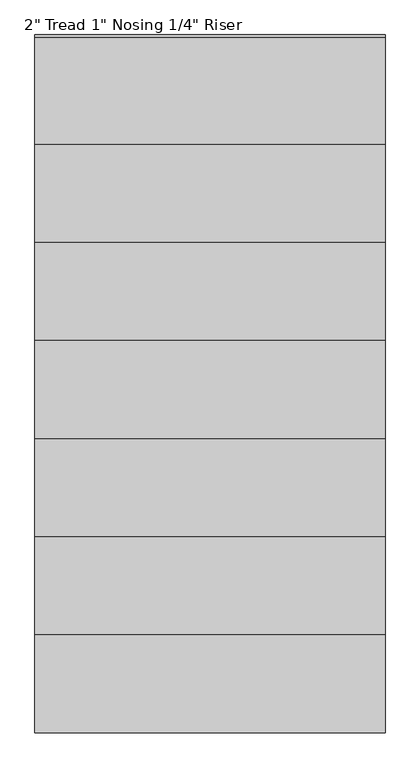
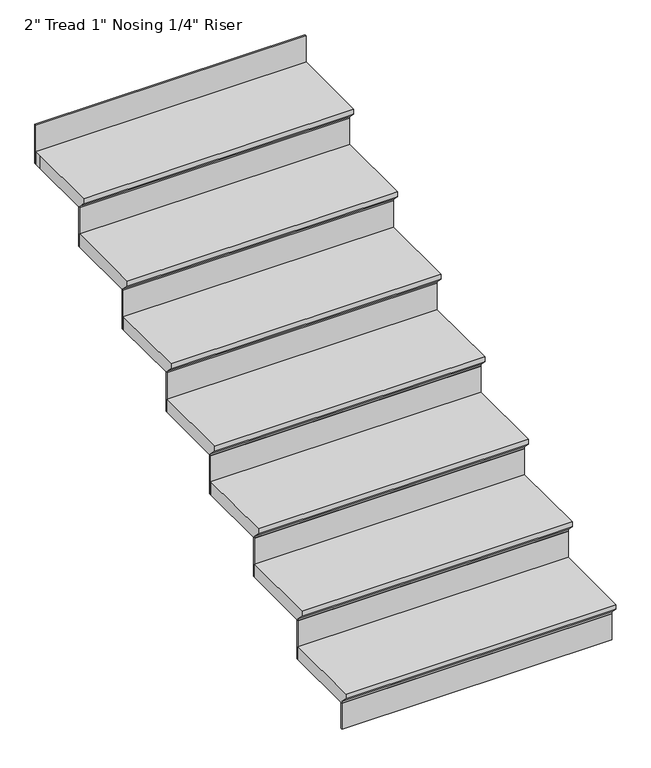
"""IFC4 building model written with IfcOpenShell, lengths in millimetres: stair flight geometry."""

from ifc_helpers import new_model, si_unit, origin, place, context, project, spatial, faceted_brep, source, transform, mapped, element, save


def stair_flight_79429955(model_context):
    return source(origin(), model_context, "Body", "Brep", [
        faceted_brep([(-6818.6502526, 9239.7128362, 133.35), (-6818.6502526, 9239.7128362, 152.4), (-7815.6002526, 9239.7128362, 152.4), (-7815.6002526, 9239.7128362, 133.35), (-6818.6502526, 9265.1128362, 107.95), (-7815.6002526, 9265.1128362, 107.95), (-6818.6502526, 9544.5128362, 152.4), (-7815.6002526, 9544.5128362, 152.4), (-7815.6002526, 9265.1128362, 101.6), (-7815.6002526, 9544.5128362, 101.6), (-6818.6502526, 9544.5128362, 101.6), (-6818.6502526, 9265.1128362, 101.6)], [[[0, 1, 2, 3]], [[4, 0, 3, 5]], [[2, 1, 6, 7]], [[8, 9, 10, 11]], [[2, 7, 9, 8, 5, 3]], [[8, 11, 4, 5]], [[6, 1, 0, 4, 11, 10]], [[7, 6, 10, 9]]]),
        faceted_brep([(-6818.6502526, 9265.1128362, 101.6), (-6818.6502526, 9265.1128362, 0.0), (-6818.6502526, 9271.4628362, 0.0), (-6818.6502526, 9271.4628362, 101.6), (-7815.6002526, 9265.1128362, 101.6), (-7815.6002526, 9271.4628362, 101.6), (-7815.6002526, 9271.4628362, 0.0), (-7815.6002526, 9265.1128362, 0.0)], [[[0, 1, 2, 3]], [[4, 5, 6, 7]], [[1, 0, 4, 7]], [[2, 1, 7, 6]], [[3, 2, 6, 5]], [[0, 3, 5, 4]]]),
        faceted_brep([(-6818.6502526, 9544.5128362, 254.0), (-6818.6502526, 9544.5128362, 101.6), (-6818.6502526, 9550.8628362, 101.6), (-6818.6502526, 9550.8628362, 254.0), (-7815.6002526, 9544.5128362, 254.0), (-7815.6002526, 9550.8628362, 254.0), (-7815.6002526, 9550.8628362, 101.6), (-7815.6002526, 9544.5128362, 101.6)], [[[0, 1, 2, 3]], [[4, 5, 6, 7]], [[1, 0, 4, 7]], [[2, 1, 7, 6]], [[3, 2, 6, 5]], [[0, 3, 5, 4]]]),
        faceted_brep([(-7815.6002526, 9519.1128362, 304.8), (-6818.6502526, 9519.1128362, 304.8), (-6818.6502526, 9823.9128362, 304.8), (-7815.6002526, 9823.9128362, 304.8), (-7815.6002526, 9544.5128362, 254.0), (-7815.6002526, 9823.9128362, 254.0), (-6818.6502526, 9823.9128362, 254.0), (-6818.6502526, 9544.5128362, 254.0), (-7815.6002526, 9544.5128362, 260.35), (-7815.6002526, 9519.1128362, 285.75), (-6818.6502526, 9544.5128362, 260.35), (-6818.6502526, 9519.1128362, 285.75)], [[[0, 1, 2, 3]], [[4, 5, 6, 7]], [[0, 3, 5, 4, 8, 9]], [[4, 7, 10, 8]], [[2, 1, 11, 10, 7, 6]], [[3, 2, 6, 5]], [[11, 1, 0, 9]], [[10, 11, 9, 8]]]),
        faceted_brep([(-6818.6502526, 9823.9128362, 406.4), (-6818.6502526, 9823.9128362, 254.0), (-6818.6502526, 9830.2628362, 254.0), (-6818.6502526, 9830.2628362, 406.4), (-7815.6002526, 9823.9128362, 406.4), (-7815.6002526, 9830.2628362, 406.4), (-7815.6002526, 9830.2628362, 254.0), (-7815.6002526, 9823.9128362, 254.0)], [[[0, 1, 2, 3]], [[4, 5, 6, 7]], [[1, 0, 4, 7]], [[2, 1, 7, 6]], [[3, 2, 6, 5]], [[0, 3, 5, 4]]]),
        faceted_brep([(-7815.6002526, 9798.5128362, 457.2), (-6818.6502526, 9798.5128362, 457.2), (-6818.6502526, 10103.3128362, 457.2), (-7815.6002526, 10103.3128362, 457.2), (-7815.6002526, 9823.9128362, 406.4), (-7815.6002526, 10103.3128362, 406.4), (-6818.6502526, 10103.3128362, 406.4), (-6818.6502526, 9823.9128362, 406.4), (-7815.6002526, 9823.9128362, 412.75), (-7815.6002526, 9798.5128362, 438.15), (-6818.6502526, 9823.9128362, 412.75), (-6818.6502526, 9798.5128362, 438.15)], [[[0, 1, 2, 3]], [[4, 5, 6, 7]], [[0, 3, 5, 4, 8, 9]], [[4, 7, 10, 8]], [[2, 1, 11, 10, 7, 6]], [[3, 2, 6, 5]], [[11, 1, 0, 9]], [[10, 11, 9, 8]]]),
        faceted_brep([(-6818.6502526, 10103.3128362, 558.8), (-6818.6502526, 10103.3128362, 406.4), (-6818.6502526, 10109.6628362, 406.4), (-6818.6502526, 10109.6628362, 558.8), (-7815.6002526, 10103.3128362, 558.8), (-7815.6002526, 10109.6628362, 558.8), (-7815.6002526, 10109.6628362, 406.4), (-7815.6002526, 10103.3128362, 406.4)], [[[0, 1, 2, 3]], [[4, 5, 6, 7]], [[1, 0, 4, 7]], [[2, 1, 7, 6]], [[3, 2, 6, 5]], [[0, 3, 5, 4]]]),
        faceted_brep([(-7815.6002526, 10077.9128362, 609.6), (-6818.6502526, 10077.9128362, 609.6), (-6818.6502526, 10382.7128362, 609.6), (-7815.6002526, 10382.7128362, 609.6), (-7815.6002526, 10103.3128362, 558.8), (-7815.6002526, 10382.7128362, 558.8), (-6818.6502526, 10382.7128362, 558.8), (-6818.6502526, 10103.3128362, 558.8), (-7815.6002526, 10103.3128362, 565.15), (-7815.6002526, 10077.9128362, 590.55), (-6818.6502526, 10103.3128362, 565.15), (-6818.6502526, 10077.9128362, 590.55)], [[[0, 1, 2, 3]], [[4, 5, 6, 7]], [[0, 3, 5, 4, 8, 9]], [[4, 7, 10, 8]], [[2, 1, 11, 10, 7, 6]], [[3, 2, 6, 5]], [[11, 1, 0, 9]], [[10, 11, 9, 8]]]),
        faceted_brep([(-6818.6502526, 10382.7128362, 711.2), (-6818.6502526, 10382.7128362, 558.8), (-6818.6502526, 10389.0628362, 558.8), (-6818.6502526, 10389.0628362, 711.2), (-7815.6002526, 10382.7128362, 711.2), (-7815.6002526, 10389.0628362, 711.2), (-7815.6002526, 10389.0628362, 558.8), (-7815.6002526, 10382.7128362, 558.8)], [[[0, 1, 2, 3]], [[4, 5, 6, 7]], [[1, 0, 4, 7]], [[2, 1, 7, 6]], [[3, 2, 6, 5]], [[0, 3, 5, 4]]]),
        faceted_brep([(-7815.6002526, 10357.3128362, 762.0), (-6818.6502526, 10357.3128362, 762.0), (-6818.6502526, 10662.1128362, 762.0), (-7815.6002526, 10662.1128362, 762.0), (-7815.6002526, 10382.7128362, 711.2), (-7815.6002526, 10662.1128362, 711.2), (-6818.6502526, 10662.1128362, 711.2), (-6818.6502526, 10382.7128362, 711.2), (-7815.6002526, 10382.7128362, 717.55), (-7815.6002526, 10357.3128362, 742.95), (-6818.6502526, 10382.7128362, 717.55), (-6818.6502526, 10357.3128362, 742.95)], [[[0, 1, 2, 3]], [[4, 5, 6, 7]], [[0, 3, 5, 4, 8, 9]], [[4, 7, 10, 8]], [[2, 1, 11, 10, 7, 6]], [[3, 2, 6, 5]], [[11, 1, 0, 9]], [[10, 11, 9, 8]]]),
        faceted_brep([(-6818.6502526, 10662.1128362, 863.6), (-6818.6502526, 10662.1128362, 711.2), (-6818.6502526, 10668.4628362, 711.2), (-6818.6502526, 10668.4628362, 863.6), (-7815.6002526, 10662.1128362, 863.6), (-7815.6002526, 10668.4628362, 863.6), (-7815.6002526, 10668.4628362, 711.2), (-7815.6002526, 10662.1128362, 711.2)], [[[0, 1, 2, 3]], [[4, 5, 6, 7]], [[1, 0, 4, 7]], [[2, 1, 7, 6]], [[3, 2, 6, 5]], [[0, 3, 5, 4]]]),
        faceted_brep([(-7815.6002526, 10636.7128362, 914.4), (-6818.6502526, 10636.7128362, 914.4), (-6818.6502526, 10941.5128362, 914.4), (-7815.6002526, 10941.5128362, 914.4), (-7815.6002526, 10662.1128362, 863.6), (-7815.6002526, 10941.5128362, 863.6), (-6818.6502526, 10941.5128362, 863.6), (-6818.6502526, 10662.1128362, 863.6), (-7815.6002526, 10662.1128362, 869.95), (-7815.6002526, 10636.7128362, 895.35), (-6818.6502526, 10662.1128362, 869.95), (-6818.6502526, 10636.7128362, 895.35)], [[[0, 1, 2, 3]], [[4, 5, 6, 7]], [[0, 3, 5, 4, 8, 9]], [[4, 7, 10, 8]], [[2, 1, 11, 10, 7, 6]], [[3, 2, 6, 5]], [[11, 1, 0, 9]], [[10, 11, 9, 8]]]),
        faceted_brep([(-6818.6502526, 11220.9128362, 1168.4), (-6818.6502526, 11220.9128362, 1016.0), (-6818.6502526, 11227.2628362, 1016.0), (-6818.6502526, 11227.2628362, 1168.4), (-7815.6002526, 11220.9128362, 1168.4), (-7815.6002526, 11227.2628362, 1168.4), (-7815.6002526, 11227.2628362, 1016.0), (-7815.6002526, 11220.9128362, 1016.0)], [[[0, 1, 2, 3]], [[4, 5, 6, 7]], [[1, 0, 4, 7]], [[2, 1, 7, 6]], [[3, 2, 6, 5]], [[0, 3, 5, 4]]]),
        faceted_brep([(-6818.6502526, 10941.5128362, 1016.0), (-6818.6502526, 10941.5128362, 863.6), (-6818.6502526, 10947.8628362, 863.6), (-6818.6502526, 10947.8628362, 1016.0), (-7815.6002526, 10941.5128362, 1016.0), (-7815.6002526, 10947.8628362, 1016.0), (-7815.6002526, 10947.8628362, 863.6), (-7815.6002526, 10941.5128362, 863.6)], [[[0, 1, 2, 3]], [[4, 5, 6, 7]], [[1, 0, 4, 7]], [[2, 1, 7, 6]], [[3, 2, 6, 5]], [[0, 3, 5, 4]]]),
        faceted_brep([(-7815.6002526, 11220.9128362, 1066.8), (-7815.6002526, 11195.5128362, 1066.8), (-7815.6002526, 10916.1128362, 1066.8), (-6818.6502526, 10916.1128362, 1066.8), (-6818.6502526, 11220.9128362, 1066.8), (-7815.6002526, 11195.5128362, 1016.0), (-7815.6002526, 11220.9128362, 1016.0), (-6818.6502526, 11220.9128362, 1016.0), (-6818.6502526, 10941.5128362, 1016.0), (-7815.6002526, 10941.5128362, 1016.0), (-7815.6002526, 10941.5128362, 1022.35), (-7815.6002526, 10916.1128362, 1047.75), (-6818.6502526, 10941.5128362, 1022.35), (-6818.6502526, 10916.1128362, 1047.75)], [[[0, 1, 2, 3, 4]], [[5, 6, 7, 8, 9]], [[1, 0, 6, 5]], [[2, 1, 5, 9, 10, 11]], [[9, 8, 12, 10]], [[4, 3, 13, 12, 8, 7]], [[0, 4, 7, 6]], [[13, 3, 2, 11]], [[12, 13, 11, 10]]]),
    ])


if __name__ == "__main__":
    model = new_model("IFC4")
    model_context = context("Model", 3, world=origin())
    ifc_project = project(units=[si_unit("LENGTHUNIT", "METRE", prefix="MILLI")], contexts=[model_context])
    site = spatial("IfcSite", under=ifc_project)
    building = spatial("IfcBuilding", under=site)
    placement = place(None, origin())
    stair_flight_shape = stair_flight_79429955(model_context)
    element("IfcStairFlight", 1, ObjectType="2\" Tread 1\" Nosing 1/4\" Riser", at=placement, inside=building, context=model_context, shape_type="MappedRepresentation", body=[
        mapped(stair_flight_shape, transform((0.0, 0.0, 0.0), x_axis=(1.0, 0.0, 0.0), y_axis=(0.0, 1.0, 0.0), z_axis=(0.0, 0.0, 1.0))),
    ])
    save(model, "model.ifc")
